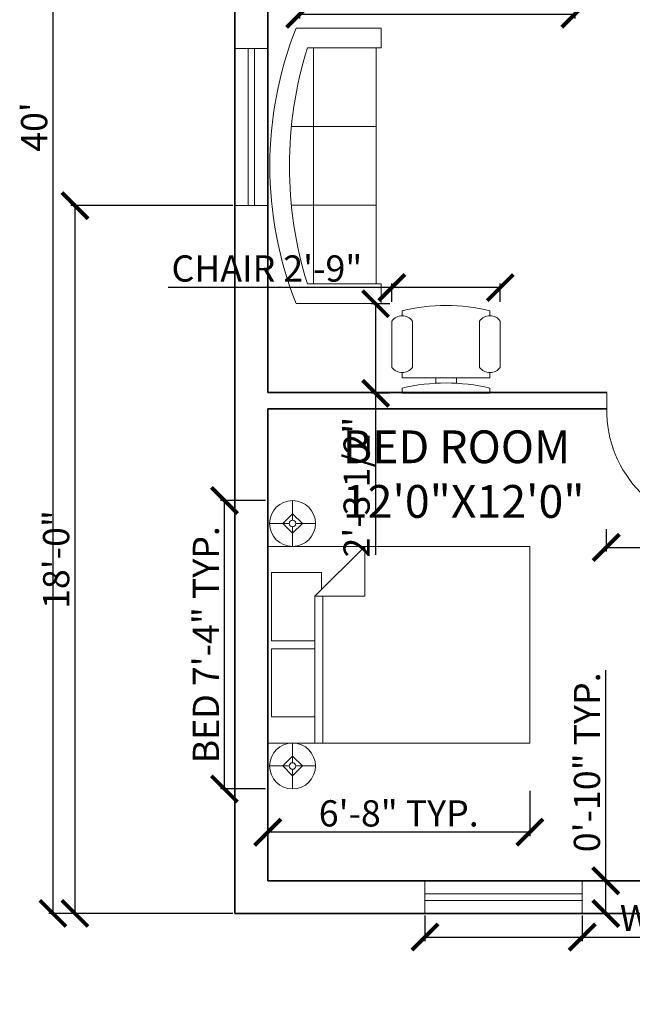
# Model space of a CAD drawing. Units: inches. Extents: x 21865 to 22885, y 36660 to 37408.
# Tile 2 of 6: x 21865 to 22052, y 36856 to 37157. Entities that reach past the tile are written whole.
import ezdxf

# ---------------------------------------------------------------- set-up
doc = ezdxf.new("R2010")
doc.units = ezdxf.units.IN
for name, color, linetype, lineweight in [('A-ANNO-DIMS', 2, 'Continuous', 18), ('A-AREA-IDEN', 7, 'Continuous', 20), ('A-DOOR', 3, 'Continuous', 20), ('A-FURN', 8, 'Continuous', 18), ('A-GLAZ', 4, 'Continuous', 18), ('A-WALL', 7, 'Continuous', 35)]:
    doc.layers.add(name, color=color, linetype=linetype, lineweight=lineweight)
doc.styles.get("Standard").update_dxf_attribs({"font": 'arial.ttf'})
doc.dimstyles.new('ISO-25', dxfattribs={"dimtxt": 8, "dimasz": 8, "dimexe": 1.25, "dimexo": 0.625, "dimtad": 1, "dimlunit": 3, "dimtxsty": 'Standard', "dimblk": 'ARCHTICK', "dimcen": 2.5, "dimclrd": 4, "dimclre": 5, "dimclrt": 1, "dimadec": 0, "dimazin": 0, "dimtfac": 1, "dimtmove": 0, "dimatfit": 3, "dimfxl": 1, "dimarcsym": 0})

# ---------------------------------------------------------------- blocks, each defined once
blk = doc.blocks.new('Bed - Queen')
for p, q in [((0, -80.00003), (0, 0)), ((0, 0), (59.99999, 0)), ((59.99999, 0), (59.99999, -80.00003)), ((7.99999, -1.2), (28.79998, -1.2)), ((7.99999, -14.4), (7.99999, -1.2)), ((28.79998, -1.2), (28.79998, -14.4)), ((31.19999, -1.2), (51.99999, -1.2)), ((31.19999, -14.4), (31.19999, -1.2)), ((51.99999, -1.2), (51.99999, -16.4)), ((0, -14.4), (44.8, -14.4)), ((59.99999, -29.6), (44.8, -14.4)), ((44.8, -14.4), (44.8, -29.6)), ((44.8, -16.8), (0, -16.8)), ((51.99999, -16.4), (46.79936, -16.4)), ((44.8, -29.6), (59.99999, -29.6)), ((59.99999, -80.00003), (0, -80.00003))]:
    blk.add_line(p, q)
blk = doc.blocks.new('Lamp - Table')
for p, q in [((0, 7), (0, 1)), ((-1, 0), (-7, 0)), ((0, 3), (-3, 0)), ((-3, 0), (0, -3)), ((3, 0), (0, 3)), ((0, -3), (3, 0)), ((1, 0), (7, 0)), ((0, -1), (0, -7))]:
    blk.add_line(p, q)
for radius in [7, 1]:
    blk.add_circle((0, 0), radius)
blk = doc.blocks.new('new block')
for name, p in [('Lamp - Table', (-35.8, -6.38)), ('Bed - Queen', (-28.8, 1.2))]:
    blk.add_blockref(name, p)
at = {"xscale": -1}
blk.add_blockref('Lamp - Table', (38.2, -6.38), dxfattribs=at)
blk = doc.blocks.new('Sofa - Roundback 7 ft.')
for p, q in [((-12.00002, -32.4421), (-12.00003, -6.5971)), ((11.99997, -32.4421), (11.99998, -6.5971)), ((-36.000027, -34), (-36.000027, -11.4696)), ((35.99998, -34), (35.99998, -11.4696)), ((-35.999844, -13.3819), (35.9998, -13.3819)), ((-36.000027, -32.4421), (35.99998, -32.4421))]:
    blk.add_line(p, q)
for points in [[(-36.000027, -34), (-42.000027, -34), (-42.000027, -8)], [(41.99998, -8), (41.99998, -34), (35.99998, -34)]]:
    blk.add_lwpolyline(points)
for centre, radius, start, end in [((0, -114.25), 114.25, 68.43141, 111.5686), ((-0.00001, -127.1968), 121.1968, 72.72033, 107.2797)]:
    blk.add_arc(centre, radius, start, end)
blk = doc.blocks.new('Chair - Desk')
for p, q in [((-8.5, 0), (-8.5, -1)), ((-8.5, 0), (8.5, 0)), ((8.5, 0), (8.5, -1)), ((-8.5, -3), (-8.5, -4)), ((-8.5, -3), (8.5, -3)), ((-2, -3), (-2, -1.9355)), ((2, -1.9576), (2, -3)), ((8.5, -3), (8.5, -4)), ((-10.5, -5), (-10.5, -14)), ((-6.5, -14), (-6.5, -5)), ((6.5, -5), (6.5, -14)), ((10.5, -14), (10.5, -5)), ((-8.5, -15), (-8.5, -16)), ((8.5, -15), (8.5, -16))]:
    blk.add_line(p, q)
for centre, radius, start, end in [((0, 34.625), 36.625, 256.5803, 283.4197), ((-8.5, -6.5), 2.5, 36.8699, 143.1301), ((8.5, -6.5), 2.5, 36.8699, 143.1301), ((-8.5, -12.5), 2.5, 216.8699, 323.1301), ((8.5, -12.5), 2.5, 216.8699, 323.1301), ((0, 19.625), 36.625, 256.5803, 283.4197)]:
    blk.add_arc(centre, radius, start, end)
blk = doc.blocks.new('_ArchTick')
at = {"color": 0, "linetype": 'ByBlock', "const_width": 0.15}
blk.add_lwpolyline([(-0.5, -0.5), (0.5, 0.5)], dxfattribs=at)
blk = doc.blocks.new('*D22')
at = {"layer": 'A-ANNO-DIMS', "color": 0, "lineweight": -2, "transparency": 16777216}
for p, q in [((21929.8, 37363.93), (21873.63, 37363.93)), ((21874.88, 37363.93), (21874.88, 36883.93)), ((21929.8, 36883.93), (21873.63, 36883.93))]:
    blk.add_line(p, q, dxfattribs=at)
at = {"layer": 'Defpoints', "color": 0, "transparency": 16777216}
for p in [(21930.43, 37363.93), (21874.88, 36883.93), (21930.43, 36883.93)]:
    blk.add_point(p, dxfattribs=at)
at = {"layer": 'A-ANNO-DIMS', "color": 0, "lineweight": -2, "transparency": 16777216, "xscale": 8, "yscale": 8, "zscale": 8}
for p, rotation in [((21874.88, 37363.93), 90), ((21874.88, 36883.93), 270)]:
    blk.add_blockref('_ArchTick', p, dxfattribs=dict(at, rotation=rotation))
at = {"layer": 'A-ANNO-DIMS', "color": 0, "transparency": 16777216, "insert": (21870.17, 37123.93), "char_height": 8, "attachment_point": 5, "rotation": 90}
blk.add_mtext("40'", dxfattribs=at)
blk = doc.blocks.new('WIN-W-48-PLAN')
for p, q in [((0, 0), (0, 10)), ((48, 0), (48, 10)), ((48, 6), (0, 6)), ((48, 4), (0, 4))]:
    blk.add_line(p, q)
blk = doc.blocks.new('DOOR-D1-36-PLAN')
for p, q in [((0, 36), (0, 41)), ((36, 36), (36, 41)), ((35, 36), (35, 0)), ((36, 36), (36, 0))]:
    blk.add_line(p, q)
blk.add_arc((35.5, 35.5), 35.5, 179.1931, 270.8069)
blk = doc.blocks.new('*D30')
at = {"layer": 'A-ANNO-DIMS', "color": 5, "lineweight": -2, "transparency": 16777216}
for p, q in [((21988.43, 36883.31), (21988.43, 36875.48)), ((22036.43, 36883.31), (22036.43, 36875.48))]:
    blk.add_line(p, q, dxfattribs=at)
at = {"layer": 'A-ANNO-DIMS', "color": 4, "lineweight": -2, "transparency": 16777216}
for p, q in [((21988.43, 36876.73), (22036.43, 36876.73)), ((22036.43, 36876.73), (22160.57, 36876.73))]:
    blk.add_line(p, q, dxfattribs=at)
at = {"layer": 'Defpoints', "color": 0, "transparency": 16777216}
for p in [(21988.43, 36883.93), (22036.43, 36883.93), (22036.43, 36876.73)]:
    blk.add_point(p, dxfattribs=at)
at = {"layer": 'A-ANNO-DIMS', "color": 4, "lineweight": -2, "transparency": 16777216, "xscale": 8, "yscale": 8, "zscale": 8, "rotation": 180}
blk.add_blockref('_ArchTick', (21988.43, 36876.73), dxfattribs=at)
at = {"layer": 'A-ANNO-DIMS', "color": 4, "lineweight": -2, "transparency": 16777216, "xscale": 8, "yscale": 8, "zscale": 8}
blk.add_blockref('_ArchTick', (22036.43, 36876.73), dxfattribs=at)
at = {"layer": 'A-ANNO-DIMS', "color": 1, "transparency": 16777216, "insert": (22102.5, 36881.5), "char_height": 8, "attachment_point": 5}
blk.add_mtext('WINDOW W 4\'-0" TYP.', dxfattribs=at)
blk = doc.blocks.new('*D31')
at = {"layer": 'A-ANNO-DIMS', "color": 4, "lineweight": -2, "transparency": 16777216}
for p, q in [((22043.63, 36893.93), (22043.63, 36958.16)), ((22043.63, 36883.93), (22043.63, 36893.93))]:
    blk.add_line(p, q, dxfattribs=at)
at = {"layer": 'A-ANNO-DIMS', "color": 5, "lineweight": -2, "transparency": 16777216}
for p, q in [((22037.05, 36893.93), (22044.88, 36893.93)), ((22037.05, 36883.93), (22044.88, 36883.93))]:
    blk.add_line(p, q, dxfattribs=at)
at = {"layer": 'Defpoints', "color": 0, "transparency": 16777216}
for p in [(22036.43, 36893.93), (22043.63, 36893.93), (22036.43, 36883.93)]:
    blk.add_point(p, dxfattribs=at)
at = {"layer": 'A-ANNO-DIMS', "color": 4, "lineweight": -2, "transparency": 16777216, "xscale": 8, "yscale": 8, "zscale": 8}
for p, rotation in [((22043.63, 36893.93), 90), ((22043.63, 36883.93), 270)]:
    blk.add_blockref('_ArchTick', p, dxfattribs=dict(at, rotation=rotation))
at = {"layer": 'A-ANNO-DIMS', "color": 1, "transparency": 16777216, "insert": (22038.92, 36930.05), "char_height": 8, "attachment_point": 5, "rotation": 90}
blk.add_mtext('0\'-10" TYP.', dxfattribs=at)
blk = doc.blocks.new('*D32')
at = {"layer": 'A-ANNO-DIMS', "color": 5, "lineweight": -2, "transparency": 16777216}
for p, q in [((21950.18, 37170.31), (21950.18, 37157.08)), ((22034.18, 37170.31), (22034.18, 37157.08))]:
    blk.add_line(p, q, dxfattribs=at)
at = {"layer": 'A-ANNO-DIMS', "color": 4, "lineweight": -2, "transparency": 16777216}
blk.add_line((21950.18, 37158.33), (22034.18, 37158.33), dxfattribs=at)
at = {"layer": 'Defpoints', "color": 0, "transparency": 16777216}
for p in [(21950.18, 37170.93), (22034.18, 37170.93), (22034.18, 37158.33)]:
    blk.add_point(p, dxfattribs=at)
at = {"layer": 'A-ANNO-DIMS', "color": 4, "lineweight": -2, "transparency": 16777216, "xscale": 8, "yscale": 8, "zscale": 8, "rotation": 180}
blk.add_blockref('_ArchTick', (21950.18, 37158.33), dxfattribs=at)
at = {"layer": 'A-ANNO-DIMS', "color": 4, "lineweight": -2, "transparency": 16777216, "xscale": 8, "yscale": 8, "zscale": 8}
blk.add_blockref('_ArchTick', (22034.18, 37158.33), dxfattribs=at)
at = {"layer": 'A-ANNO-DIMS', "color": 1, "transparency": 16777216, "insert": (21992.18, 37163.1), "char_height": 8, "attachment_point": 5}
blk.add_mtext('SOFA 7\'-0" TYP.', dxfattribs=at)
blk = doc.blocks.new('*D34')
at = {"layer": 'A-ANNO-DIMS', "color": 5, "lineweight": -2, "transparency": 16777216}
for p, q in [((21939.8, 37009.93), (21925.98, 37009.93)), ((21939.8, 36921.93), (21925.98, 36921.93))]:
    blk.add_line(p, q, dxfattribs=at)
at = {"layer": 'A-ANNO-DIMS', "color": 4, "lineweight": -2, "transparency": 16777216}
blk.add_line((21927.23, 36921.93), (21927.23, 37009.93), dxfattribs=at)
at = {"layer": 'Defpoints', "color": 0, "transparency": 16777216}
for p in [(21927.23, 37009.93), (21940.43, 37009.93), (21940.43, 36921.93)]:
    blk.add_point(p, dxfattribs=at)
at = {"layer": 'A-ANNO-DIMS', "color": 4, "lineweight": -2, "transparency": 16777216, "xscale": 8, "yscale": 8, "zscale": 8}
for p, rotation in [((21927.23, 37009.93), 90), ((21927.23, 36921.93), 270)]:
    blk.add_blockref('_ArchTick', p, dxfattribs=dict(at, rotation=rotation))
at = {"layer": 'A-ANNO-DIMS', "color": 1, "transparency": 16777216, "insert": (21922.6, 36965.93), "char_height": 8, "attachment_point": 5, "rotation": 90}
blk.add_mtext('BED 7\'-4" TYP.', dxfattribs=at)
blk = doc.blocks.new('*D35')
at = {"layer": 'A-ANNO-DIMS', "color": 5, "lineweight": -2, "transparency": 16777216}
for p, q in [((21940.43, 36921.31), (21940.43, 36907.48)), ((22020.43, 36921.31), (22020.43, 36907.48))]:
    blk.add_line(p, q, dxfattribs=at)
at = {"layer": 'A-ANNO-DIMS', "color": 4, "lineweight": -2, "transparency": 16777216}
blk.add_line((22020.43, 36908.73), (21940.43, 36908.73), dxfattribs=at)
at = {"layer": 'Defpoints', "color": 0, "transparency": 16777216}
for p in [(21940.43, 36921.93), (22020.43, 36921.93), (21940.43, 36908.73)]:
    blk.add_point(p, dxfattribs=at)
at = {"layer": 'A-ANNO-DIMS', "color": 4, "lineweight": -2, "transparency": 16777216, "xscale": 8, "yscale": 8, "zscale": 8, "rotation": 180}
blk.add_blockref('_ArchTick', (21940.43, 36908.73), dxfattribs=at)
at = {"layer": 'A-ANNO-DIMS', "color": 4, "lineweight": -2, "transparency": 16777216, "xscale": 8, "yscale": 8, "zscale": 8}
blk.add_blockref('_ArchTick', (22020.43, 36908.73), dxfattribs=at)
at = {"layer": 'A-ANNO-DIMS', "color": 1, "transparency": 16777216, "insert": (21980.43, 36913.44), "char_height": 8, "attachment_point": 5}
blk.add_mtext('6\'-8" TYP.', dxfattribs=at)
blk = doc.blocks.new('*D37')
at = {"layer": 'A-ANNO-DIMS', "color": 5, "lineweight": -2, "transparency": 16777216}
for p, q in [((22043.79, 37001.17), (22043.79, 36994.38)), ((22079.93, 37001.17), (22079.93, 36994.38))]:
    blk.add_line(p, q, dxfattribs=at)
at = {"layer": 'A-ANNO-DIMS', "color": 4, "lineweight": -2, "transparency": 16777216}
for p, q in [((22043.79, 36995.63), (22079.93, 36995.63)), ((22079.93, 36995.63), (22137.94, 36995.63))]:
    blk.add_line(p, q, dxfattribs=at)
at = {"layer": 'Defpoints', "color": 0, "transparency": 16777216}
for p in [(22043.79, 37001.8), (22079.93, 37001.8), (22079.93, 36995.63)]:
    blk.add_point(p, dxfattribs=at)
at = {"layer": 'A-ANNO-DIMS', "color": 4, "lineweight": -2, "transparency": 16777216, "xscale": 8, "yscale": 8, "zscale": 8, "rotation": 180}
blk.add_blockref('_ArchTick', (22043.79, 36995.63), dxfattribs=at)
at = {"layer": 'A-ANNO-DIMS', "color": 4, "lineweight": -2, "transparency": 16777216, "xscale": 8, "yscale": 8, "zscale": 8}
blk.add_blockref('_ArchTick', (22079.93, 36995.63), dxfattribs=at)
at = {"layer": 'A-ANNO-DIMS', "color": 1, "transparency": 16777216, "insert": (22112.93, 37000.34), "char_height": 8, "attachment_point": 5}
blk.add_mtext('3\'-0" TYP.', dxfattribs=at)
blk = doc.blocks.new('*D50')
at = {"layer": 'A-ANNO-DIMS', "color": 4, "lineweight": -2, "transparency": 16777216}
for p, q in [((21978.34, 37074.94), (21910.03, 37074.94)), ((22011.43, 37074.94), (21978.34, 37074.94))]:
    blk.add_line(p, q, dxfattribs=at)
at = {"layer": 'A-ANNO-DIMS', "color": 5, "lineweight": -2, "transparency": 16777216}
for p, q in [((21978.34, 37070.61), (21978.34, 37076.19)), ((22011.43, 37070.61), (22011.43, 37076.19))]:
    blk.add_line(p, q, dxfattribs=at)
at = {"layer": 'Defpoints', "color": 0, "transparency": 16777216}
for p in [(21978.34, 37074.94), (21978.34, 37069.98), (22011.43, 37069.98)]:
    blk.add_point(p, dxfattribs=at)
at = {"layer": 'A-ANNO-DIMS', "color": 4, "lineweight": -2, "transparency": 16777216, "xscale": 8, "yscale": 8, "zscale": 8, "rotation": 180}
blk.add_blockref('_ArchTick', (21978.34, 37074.94), dxfattribs=at)
at = {"layer": 'A-ANNO-DIMS', "color": 4, "lineweight": -2, "transparency": 16777216, "xscale": 8, "yscale": 8, "zscale": 8}
blk.add_blockref('_ArchTick', (22011.43, 37074.94), dxfattribs=at)
at = {"layer": 'A-ANNO-DIMS', "color": 1, "transparency": 16777216, "insert": (21940.18, 37079.71), "char_height": 8, "attachment_point": 5}
blk.add_mtext('CHAIR 2\'-9"', dxfattribs=at)
blk = doc.blocks.new('*D51')
at = {"layer": 'A-ANNO-DIMS', "color": 5, "lineweight": -2, "transparency": 16777216}
for p, q in [((21977.71, 37069.98), (21972.12, 37069.98)), ((21977.71, 37042.66), (21972.12, 37042.66))]:
    blk.add_line(p, q, dxfattribs=at)
at = {"layer": 'A-ANNO-DIMS', "color": 4, "lineweight": -2, "transparency": 16777216}
for p, q in [((21973.37, 37069.98), (21973.37, 37042.66)), ((21973.37, 37042.66), (21973.37, 36993.37))]:
    blk.add_line(p, q, dxfattribs=at)
at = {"layer": 'Defpoints', "color": 0, "transparency": 16777216}
for p in [(21978.34, 37069.98), (21973.37, 37042.66), (21978.34, 37042.66)]:
    blk.add_point(p, dxfattribs=at)
at = {"layer": 'A-ANNO-DIMS', "color": 4, "lineweight": -2, "transparency": 16777216, "xscale": 8, "yscale": 8, "zscale": 8}
for p, rotation in [((21973.37, 37069.98), 90), ((21973.37, 37042.66), 270)]:
    blk.add_blockref('_ArchTick', p, dxfattribs=dict(at, rotation=rotation))
at = {"layer": 'A-ANNO-DIMS', "color": 1, "transparency": 16777216, "insert": (21968.61, 37014.02), "char_height": 8, "attachment_point": 5, "rotation": 90}
blk.add_mtext('2\'-3 1/2"', dxfattribs=at)
blk = doc.blocks.new('*D55')
at = {"layer": 'A-ANNO-DIMS', "color": 5, "lineweight": -2, "transparency": 16777216}
for p, q in [((21929.8, 37099.93), (21880.34, 37099.93)), ((21929.8, 36883.93), (21880.34, 36883.93))]:
    blk.add_line(p, q, dxfattribs=at)
at = {"layer": 'A-ANNO-DIMS', "color": 4, "lineweight": -2, "transparency": 16777216}
blk.add_line((21881.59, 37099.93), (21881.59, 36883.93), dxfattribs=at)
at = {"layer": 'Defpoints', "color": 0, "transparency": 16777216}
for p in [(21930.43, 37099.93), (21881.59, 36883.93), (21930.43, 36883.93)]:
    blk.add_point(p, dxfattribs=at)
at = {"layer": 'A-ANNO-DIMS', "color": 4, "lineweight": -2, "transparency": 16777216, "xscale": 8, "yscale": 8, "zscale": 8}
for p, rotation in [((21881.59, 37099.93), 90), ((21881.59, 36883.93), 270)]:
    blk.add_blockref('_ArchTick', p, dxfattribs=dict(at, rotation=rotation))
at = {"layer": 'A-ANNO-DIMS', "color": 1, "transparency": 16777216, "insert": (21876.88, 36991.93), "char_height": 8, "attachment_point": 5, "rotation": 90}
blk.add_mtext('18\'-0"', dxfattribs=at)

msp = doc.modelspace()

# ---------------------------------------------------------------- linework, layer by layer
at = {"layer": 'A-WALL'}
for p, q in [((21930.43, 36883.931), (21930.43, 37363.931)), ((21940.43, 37042.931), (21940.43, 37204.931)), ((22043.93, 37042.931), (21940.43, 37042.931)), ((21940.43, 36893.931), (21940.43, 37037.931)), ((22043.93, 37037.931), (21940.43, 37037.931)), ((22043.93, 37037.931), (21940.43, 37037.931)), ((22084.43, 36893.931), (21940.43, 36893.931)), ((22089.43, 36883.931), (21930.43, 36883.931))]:
    msp.add_line(p, q, dxfattribs=at)

# ---------------------------------------------------------------- block references
at = {"layer": 'A-DOOR'}
msp.add_blockref('DOOR-D1-36-PLAN', (22043.929, 37001.93), dxfattribs=at)
at = {"layer": 'A-FURN', "rotation": 90}
for name, p in [('Sofa - Roundback 7 ft.', (21941.075, 37112.053)), ('new block', (21941.63, 36964.731))]:
    msp.add_blockref(name, p, dxfattribs=at)
at = {"layer": 'A-FURN', "xscale": 1.576046386133933, "yscale": 1.576046386133933, "zscale": 1.576046386133933, "rotation": 180}
msp.add_blockref('Chair - Desk', (21994.884, 37042.662), dxfattribs=at)
at = {"layer": 'A-GLAZ', "rotation": 89.99999999998334}
msp.add_blockref('WIN-W-48-PLAN', (21940.43, 37099.932), dxfattribs=at)
at = {"layer": 'A-GLAZ'}
msp.add_blockref('WIN-W-48-PLAN', (21988.43, 36883.931), dxfattribs=at)

# ---------------------------------------------------------------- texts
at = {"layer": 'A-AREA-IDEN', "insert": (21963.37, 37031.339), "char_height": 10, "attachment_point": 1}
msp.add_mtext_dynamic_manual_height_columns('BED ROOM\\P12\'0"X12\'0"', width=146.69061, gutter_width=12.5, heights=[0], dxfattribs=at)

# ---------------------------------------------------------------- dimensions: what is measured, and where the dimension line sits
at = {"layer": 'A-ANNO-DIMS'}
for base, p1, p2, angle, override, picture, middle in [((21874.88, 36883.931), (21930.43, 37363.931), (21930.43, 36883.931), 90, {"dimclrd": 0, "dimclre": 0, "dimclrt": 0}, '*D22', (21870.171, 37123.931)), ((21881.59, 36883.931), (21930.43, 37099.931), (21930.43, 36883.931), 90, {"dimdec": 1, "dimlfac": 1, "dimrnd": 0, "dimzin": 1, "dimdsep": 46, "dimlunit": 4, "dimfrac": 2}, '*D55', (21876.881, 36991.931)), ((21973.371, 37042.662), (21978.335, 37069.98), (21978.335, 37042.662), 270, {"dimdec": 1, "dimlfac": 1, "dimrnd": 0, "dimzin": 1, "dimdsep": 46, "dimlunit": 4, "dimfrac": 2}, '*D51', (21968.606, 37014.015))]:
    dim = msp.add_linear_dim(base=base, p1=p1, p2=p2, angle=angle, dimstyle='ISO-25', override=override, dxfattribs=at)
    dim.commit()
    dim.dimension.update_dxf_attribs({"geometry": picture, "text_midpoint": middle})
for base, p1, p2, text, picture, middle in [((22034.18, 37158.331), (21950.18, 37170.931), (22034.18, 37170.931), 'SOFA <> TYP.', '*D32', (21992.18, 37163.096)), ((22079.93, 36995.626), (22043.795, 37001.796), (22079.93, 37001.796), '<> TYP.', '*D37', (22112.934, 37000.338)), ((22036.43, 36876.731), (21988.43, 36883.931), (22036.43, 36883.931), 'WINDOW W <> TYP.', '*D30', (22102.498, 36881.496))]:
    dim = msp.add_linear_dim(base=base, p1=p1, p2=p2, text=text, dimstyle='ISO-25', override={"dimdec": 1, "dimlfac": 1, "dimrnd": 0, "dimzin": 1, "dimdsep": 46, "dimlunit": 4, "dimfrac": 2}, dxfattribs=at)
    dim.commit()
    dim.dimension.update_dxf_attribs({"geometry": picture, "text_midpoint": middle})
for base, p1, p2, angle, text, picture, middle in [((21978.335, 37074.945), (22011.432, 37069.98), (21978.335, 37069.98), 180, 'CHAIR <>', '*D50', (21940.185, 37079.706)), ((21927.23, 37009.931), (21940.43, 36921.931), (21940.43, 37009.931), 90, 'BED <> TYP.', '*D34', (21922.602, 36965.931)), ((22043.63, 36893.931), (22036.43, 36883.931), (22036.43, 36893.931), 90, '<> TYP.', '*D31', (22038.92, 36930.046)), ((21940.43, 36908.731), (22020.43, 36921.931), (21940.43, 36921.931), 180, '<> TYP.', '*D35', (21980.43, 36913.441))]:
    dim = msp.add_linear_dim(base=base, p1=p1, p2=p2, angle=angle, text=text, dimstyle='ISO-25', override={"dimdec": 1, "dimlfac": 1, "dimrnd": 0, "dimzin": 1, "dimdsep": 46, "dimlunit": 4, "dimfrac": 2}, dxfattribs=at)
    dim.commit()
    dim.dimension.update_dxf_attribs({"geometry": picture, "text_midpoint": middle})

doc.saveas('drawing.dxf')
